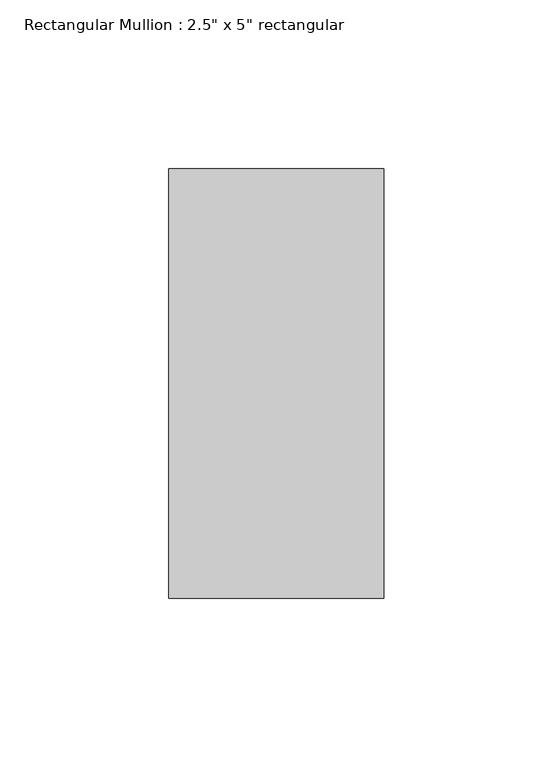
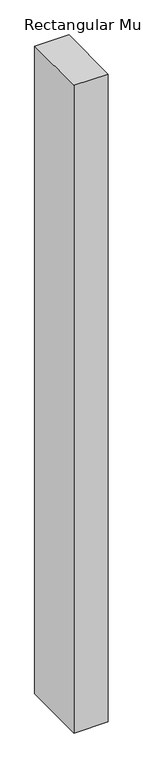
"""IFC4 building model written with IfcOpenShell, lengths in millimetres: member geometry."""

from ifc_helpers import new_model, si_unit, frame, origin, place, context, project, spatial, polyline, outline, extrude, source, transform, mapped, element, save


def member_87553b7f(model_context):
    return source(origin(), model_context, "Body", "SweptSolid", [
        extrude(outline(polyline([(0.0, 63.5), (0.0, -63.5), (-63.5, -63.5), (-63.5, 63.5), (0.0, 63.5)])), frame((0.0, 0.0, -1273.4060005), z_axis=(0.0, 0.0, 1.0), x_axis=(1.0, 0.0, 0.0)), (0.0, 0.0, 1.0), 1273.4060005),
    ])


if __name__ == "__main__":
    model = new_model("IFC4")
    model_context = context("Model", 3, world=origin())
    ifc_project = project(units=[si_unit("LENGTHUNIT", "METRE", prefix="MILLI")], contexts=[model_context])
    site = spatial("IfcSite", under=ifc_project)
    building = spatial("IfcBuilding", under=site)
    placement = place(None, origin())
    member_shape = member_87553b7f(model_context)
    element("IfcMember", 1, ObjectType="Rectangular Mullion : 2.5\" x 5\" rectangular", at=placement, inside=building, context=model_context, shape_type="MappedRepresentation", body=[
        mapped(member_shape, transform((0.0, 0.0, 0.0), x_axis=(1.0, 0.0, 0.0), y_axis=(0.0, 1.0, 0.0), z_axis=(0.0, 0.0, 1.0))),
    ])
    save(model, "model.ifc")

# Revit data of these elements
# Type "Rectangular Mullion : 2.5\" x 5\" rectangular"
#   built-in parameter 1007304 = 0.416667 (stored number, unit not read)
#   built-in parameter 1007301 = 0.104167 (stored number, unit not read)
#   built-in parameter 1007300 = 0.104167 (stored number, unit not read)
# Element 1 (IfcMember, "Rectangular Mullion : 2.5\" x 5\" rectangular")
#   Materials on its faces: "Aluminum"
# Materials
#   "Aluminum": class "Metal", colour RGB 247 247 247, transparency 0, Description = "Aluminum 6061", Cost = 0
